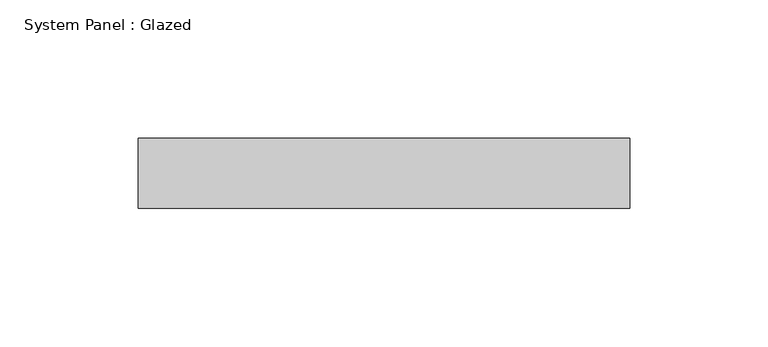
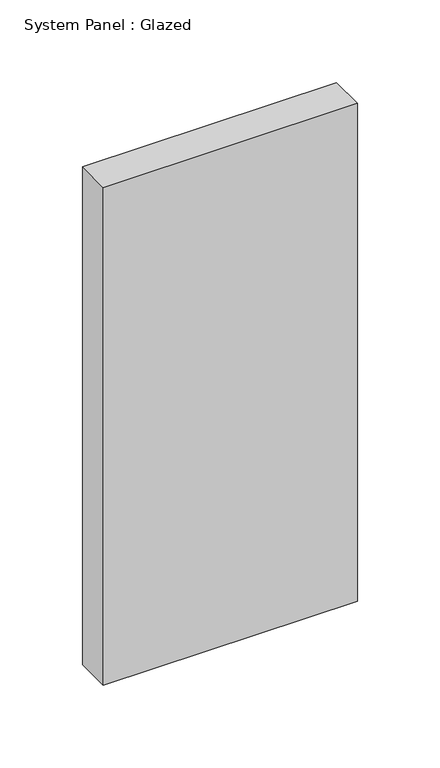
"""IFC4 building model written with IfcOpenShell, lengths in millimetres: plate geometry, System Panel : Glazed."""

from ifc_helpers import new_model, si_unit, origin, origin_with_axes, place, context, project, spatial, polyline, outline, extrude, source, transform, mapped, element, save


def system_panel_glazed_d1623790(model_context):
    return source(origin(), model_context, "Body", "SweptSolid", [
        extrude(outline(polyline([(88.9, 19.05), (-88.9, 19.05), (-88.9, 44.45), (88.9, 44.45), (88.9, 19.05)])), origin_with_axes(), (0.0, 0.0, 1.0), 368.3),
    ])


if __name__ == "__main__":
    model = new_model("IFC4")
    model_context = context("Model", 3, world=origin())
    ifc_project = project(units=[si_unit("LENGTHUNIT", "METRE", prefix="MILLI")], contexts=[model_context])
    site = spatial("IfcSite", under=ifc_project)
    building = spatial("IfcBuilding", under=site)
    placement = place(None, origin())
    system_panel_glazed_shape = system_panel_glazed_d1623790(model_context)
    element("IfcPlate", 1, ObjectType="System Panel : Glazed", at=placement, inside=building, context=model_context, shape_type="MappedRepresentation", body=[
        mapped(system_panel_glazed_shape, transform((0.0, 0.0, 0.0), x_axis=(1.0, 0.0, 0.0), y_axis=(0.0, 1.0, 0.0), z_axis=(0.0, 0.0, 1.0))),
    ])
    save(model, "model.ifc")

# Revit data of these elements
# Type "System Panel : Glazed"
#   Construction Type Id = "GSP4R"
#   Analytic Construction = "1/8 in Pilkington single glazing"
#   Visual Light Transmittance = 0.9
#   Solar Heat Gain Coefficient = 0.86
#   Heat Transfer Coefficient (U) = 1.18115 BTU/(h·ft²·°F)
#   Define Thermal Properties by = 1
# Element 1 (IfcPlate, "System Panel : Glazed")
#   Materials on its faces: "Glass"
# Materials
#   "Glass": class "Glass", colour RGB 0 128 192, transparency 0.75, Description = "Soda Lime Glass", Cost = 0
